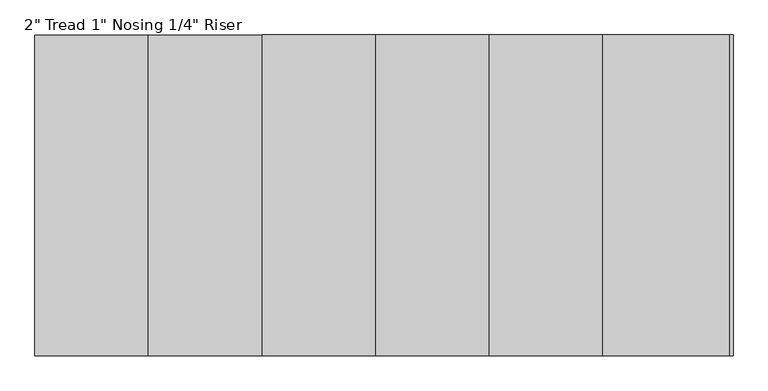
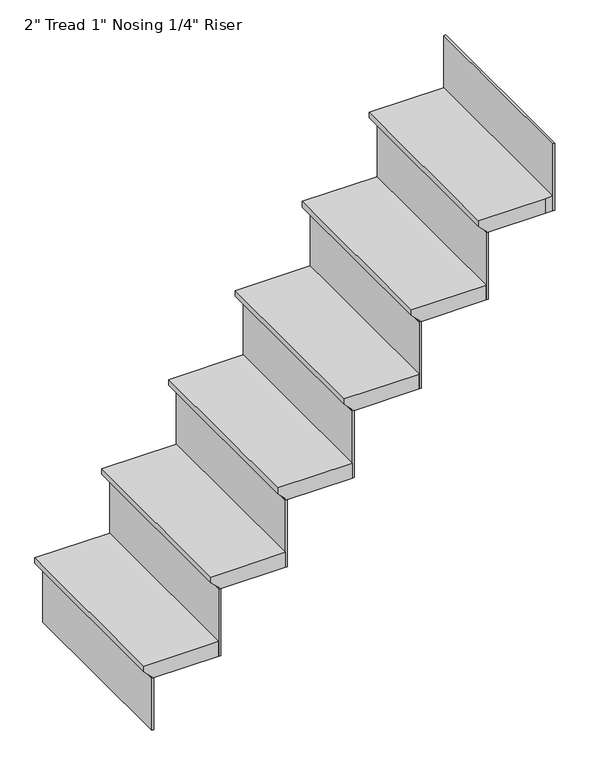
"""IFC4 building model written with IfcOpenShell, lengths in millimetres: stair flight geometry."""

from ifc_helpers import new_model, si_unit, origin, place, context, project, spatial, faceted_brep, source, transform, mapped, element, save


def stair_flight_48b2ccee(model_context):
    return source(origin(), model_context, "Body", "Brep", [
        faceted_brep([(-4591.4237097, 3724.9480625, 3409.95), (-4591.4237097, 3724.9480625, 3429.0), (-4591.4237097, 4334.5480625, 3429.0), (-4591.4237097, 4334.5480625, 3409.95), (-4566.0237097, 3724.9480625, 3384.55), (-4566.0237097, 4334.5480625, 3384.55), (-4350.1237097, 3724.9480625, 3429.0), (-4350.1237097, 4334.5480625, 3429.0), (-4566.0237097, 4334.5480625, 3378.2), (-4350.1237097, 4334.5480625, 3378.2), (-4350.1237097, 3724.9480625, 3378.2), (-4566.0237097, 3724.9480625, 3378.2)], [[[0, 1, 2, 3]], [[4, 0, 3, 5]], [[2, 1, 6, 7]], [[8, 9, 10, 11]], [[2, 7, 9, 8, 5, 3]], [[8, 11, 4, 5]], [[6, 1, 0, 4, 11, 10]], [[7, 6, 10, 9]]]),
        faceted_brep([(-4566.0237097, 3724.9480625, 3378.2), (-4566.0237097, 3724.9480625, 3200.4), (-4559.6737097, 3724.9480625, 3200.4), (-4559.6737097, 3724.9480625, 3378.2), (-4566.0237097, 4334.5480625, 3378.2), (-4559.6737097, 4334.5480625, 3378.2), (-4559.6737097, 4334.5480625, 3200.4), (-4566.0237097, 4334.5480625, 3200.4)], [[[0, 1, 2, 3]], [[4, 5, 6, 7]], [[1, 0, 4, 7]], [[2, 1, 7, 6]], [[3, 2, 6, 5]], [[0, 3, 5, 4]]]),
        faceted_brep([(-3270.6237097, 3724.9480625, 4749.8), (-3270.6237097, 3724.9480625, 4521.2), (-3264.2737097, 3724.9480625, 4521.2), (-3264.2737097, 3724.9480625, 4749.8), (-3270.6237097, 4334.5480625, 4749.8), (-3264.2737097, 4334.5480625, 4749.8), (-3264.2737097, 4334.5480625, 4521.2), (-3270.6237097, 4334.5480625, 4521.2)], [[[0, 1, 2, 3]], [[4, 5, 6, 7]], [[1, 0, 4, 7]], [[2, 1, 7, 6]], [[3, 2, 6, 5]], [[0, 3, 5, 4]]]),
        faceted_brep([(-4350.1237097, 3724.9480625, 3606.8), (-4350.1237097, 3724.9480625, 3378.2), (-4343.7737097, 3724.9480625, 3378.2), (-4343.7737097, 3724.9480625, 3606.8), (-4350.1237097, 4334.5480625, 3606.8), (-4343.7737097, 4334.5480625, 3606.8), (-4343.7737097, 4334.5480625, 3378.2), (-4350.1237097, 4334.5480625, 3378.2)], [[[0, 1, 2, 3]], [[4, 5, 6, 7]], [[1, 0, 4, 7]], [[2, 1, 7, 6]], [[3, 2, 6, 5]], [[0, 3, 5, 4]]]),
        faceted_brep([(-4375.5237097, 4334.5480625, 3657.6), (-4375.5237097, 3724.9480625, 3657.6), (-4134.2237097, 3724.9480625, 3657.6), (-4134.2237097, 4334.5480625, 3657.6), (-4350.1237097, 4334.5480625, 3606.8), (-4134.2237097, 4334.5480625, 3606.8), (-4134.2237097, 3724.9480625, 3606.8), (-4350.1237097, 3724.9480625, 3606.8), (-4350.1237097, 4334.5480625, 3613.15), (-4375.5237097, 4334.5480625, 3638.55), (-4350.1237097, 3724.9480625, 3613.15), (-4375.5237097, 3724.9480625, 3638.55)], [[[0, 1, 2, 3]], [[4, 5, 6, 7]], [[0, 3, 5, 4, 8, 9]], [[4, 7, 10, 8]], [[2, 1, 11, 10, 7, 6]], [[3, 2, 6, 5]], [[11, 1, 0, 9]], [[10, 11, 9, 8]]]),
        faceted_brep([(-4134.2237097, 3724.9480625, 3835.4), (-4134.2237097, 3724.9480625, 3606.8), (-4127.8737097, 3724.9480625, 3606.8), (-4127.8737097, 3724.9480625, 3835.4), (-4134.2237097, 4334.5480625, 3835.4), (-4127.8737097, 4334.5480625, 3835.4), (-4127.8737097, 4334.5480625, 3606.8), (-4134.2237097, 4334.5480625, 3606.8)], [[[0, 1, 2, 3]], [[4, 5, 6, 7]], [[1, 0, 4, 7]], [[2, 1, 7, 6]], [[3, 2, 6, 5]], [[0, 3, 5, 4]]]),
        faceted_brep([(-4159.6237097, 4334.5480625, 3886.2), (-4159.6237097, 3724.9480625, 3886.2), (-3918.3237097, 3724.9480625, 3886.2), (-3918.3237097, 4334.5480625, 3886.2), (-4134.2237097, 4334.5480625, 3835.4), (-3918.3237097, 4334.5480625, 3835.4), (-3918.3237097, 3724.9480625, 3835.4), (-4134.2237097, 3724.9480625, 3835.4), (-4134.2237097, 4334.5480625, 3841.75), (-4159.6237097, 4334.5480625, 3867.15), (-4134.2237097, 3724.9480625, 3841.75), (-4159.6237097, 3724.9480625, 3867.15)], [[[0, 1, 2, 3]], [[4, 5, 6, 7]], [[0, 3, 5, 4, 8, 9]], [[4, 7, 10, 8]], [[2, 1, 11, 10, 7, 6]], [[3, 2, 6, 5]], [[11, 1, 0, 9]], [[10, 11, 9, 8]]]),
        faceted_brep([(-3918.3237097, 3724.9480625, 4064.0), (-3918.3237097, 3724.9480625, 3835.4), (-3911.9737097, 3724.9480625, 3835.4), (-3911.9737097, 3724.9480625, 4064.0), (-3918.3237097, 4334.5480625, 4064.0), (-3911.9737097, 4334.5480625, 4064.0), (-3911.9737097, 4334.5480625, 3835.4), (-3918.3237097, 4334.5480625, 3835.4)], [[[0, 1, 2, 3]], [[4, 5, 6, 7]], [[1, 0, 4, 7]], [[2, 1, 7, 6]], [[3, 2, 6, 5]], [[0, 3, 5, 4]]]),
        faceted_brep([(-3943.7237097, 4334.5480625, 4114.8), (-3943.7237097, 3724.9480625, 4114.8), (-3702.4237097, 3724.9480625, 4114.8), (-3702.4237097, 4334.5480625, 4114.8), (-3918.3237097, 4334.5480625, 4064.0), (-3702.4237097, 4334.5480625, 4064.0), (-3702.4237097, 3724.9480625, 4064.0), (-3918.3237097, 3724.9480625, 4064.0), (-3918.3237097, 4334.5480625, 4070.35), (-3943.7237097, 4334.5480625, 4095.75), (-3918.3237097, 3724.9480625, 4070.35), (-3943.7237097, 3724.9480625, 4095.75)], [[[0, 1, 2, 3]], [[4, 5, 6, 7]], [[0, 3, 5, 4, 8, 9]], [[4, 7, 10, 8]], [[2, 1, 11, 10, 7, 6]], [[3, 2, 6, 5]], [[11, 1, 0, 9]], [[10, 11, 9, 8]]]),
        faceted_brep([(-3702.4237097, 3724.9480625, 4292.6), (-3702.4237097, 3724.9480625, 4064.0), (-3696.0737097, 3724.9480625, 4064.0), (-3696.0737097, 3724.9480625, 4292.6), (-3702.4237097, 4334.5480625, 4292.6), (-3696.0737097, 4334.5480625, 4292.6), (-3696.0737097, 4334.5480625, 4064.0), (-3702.4237097, 4334.5480625, 4064.0)], [[[0, 1, 2, 3]], [[4, 5, 6, 7]], [[1, 0, 4, 7]], [[2, 1, 7, 6]], [[3, 2, 6, 5]], [[0, 3, 5, 4]]]),
        faceted_brep([(-3727.8237097, 4334.5480625, 4343.4), (-3727.8237097, 3724.9480625, 4343.4), (-3486.5237097, 3724.9480625, 4343.4), (-3486.5237097, 4334.5480625, 4343.4), (-3702.4237097, 4334.5480625, 4292.6), (-3486.5237097, 4334.5480625, 4292.6), (-3486.5237097, 3724.9480625, 4292.6), (-3702.4237097, 3724.9480625, 4292.6), (-3702.4237097, 4334.5480625, 4298.95), (-3727.8237097, 4334.5480625, 4324.35), (-3702.4237097, 3724.9480625, 4298.95), (-3727.8237097, 3724.9480625, 4324.35)], [[[0, 1, 2, 3]], [[4, 5, 6, 7]], [[0, 3, 5, 4, 8, 9]], [[4, 7, 10, 8]], [[2, 1, 11, 10, 7, 6]], [[3, 2, 6, 5]], [[11, 1, 0, 9]], [[10, 11, 9, 8]]]),
        faceted_brep([(-3486.5237097, 3724.9480625, 4521.2), (-3486.5237097, 3724.9480625, 4292.6), (-3480.1737097, 3724.9480625, 4292.6), (-3480.1737097, 3724.9480625, 4521.2), (-3486.5237097, 4334.5480625, 4521.2), (-3480.1737097, 4334.5480625, 4521.2), (-3480.1737097, 4334.5480625, 4292.6), (-3486.5237097, 4334.5480625, 4292.6)], [[[0, 1, 2, 3]], [[4, 5, 6, 7]], [[1, 0, 4, 7]], [[2, 1, 7, 6]], [[3, 2, 6, 5]], [[0, 3, 5, 4]]]),
        faceted_brep([(-3511.9237097, 4334.5480625, 4572.0), (-3511.9237097, 3724.9480625, 4572.0), (-3296.0237097, 3724.9480625, 4572.0), (-3270.6237097, 3724.9480625, 4572.0), (-3270.6237097, 4334.5480625, 4572.0), (-3486.5237097, 4334.5480625, 4521.2), (-3270.6237097, 4334.5480625, 4521.2), (-3270.6237097, 3724.9480625, 4521.2), (-3296.0237097, 3724.9480625, 4521.2), (-3486.5237097, 3724.9480625, 4521.2), (-3486.5237097, 4334.5480625, 4527.55), (-3511.9237097, 4334.5480625, 4552.95), (-3486.5237097, 3724.9480625, 4527.55), (-3511.9237097, 3724.9480625, 4552.95)], [[[0, 1, 2, 3, 4]], [[5, 6, 7, 8, 9]], [[0, 4, 6, 5, 10, 11]], [[5, 9, 12, 10]], [[2, 1, 13, 12, 9, 8]], [[3, 2, 8, 7]], [[4, 3, 7, 6]], [[13, 1, 0, 11]], [[12, 13, 11, 10]]]),
    ])


if __name__ == "__main__":
    model = new_model("IFC4")
    model_context = context("Model", 3, world=origin())
    ifc_project = project(units=[si_unit("LENGTHUNIT", "METRE", prefix="MILLI")], contexts=[model_context])
    site = spatial("IfcSite", under=ifc_project)
    building = spatial("IfcBuilding", under=site)
    placement = place(None, origin())
    stair_flight_shape = stair_flight_48b2ccee(model_context)
    element("IfcStairFlight", 1, ObjectType="2\" Tread 1\" Nosing 1/4\" Riser", at=placement, inside=building, context=model_context, shape_type="MappedRepresentation", body=[
        mapped(stair_flight_shape, transform((0.0, 0.0, 0.0), x_axis=(1.0, 0.0, 0.0), y_axis=(0.0, 1.0, 0.0), z_axis=(0.0, 0.0, 1.0))),
    ])
    save(model, "model.ifc")
